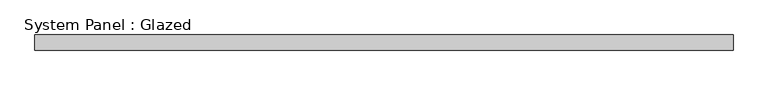
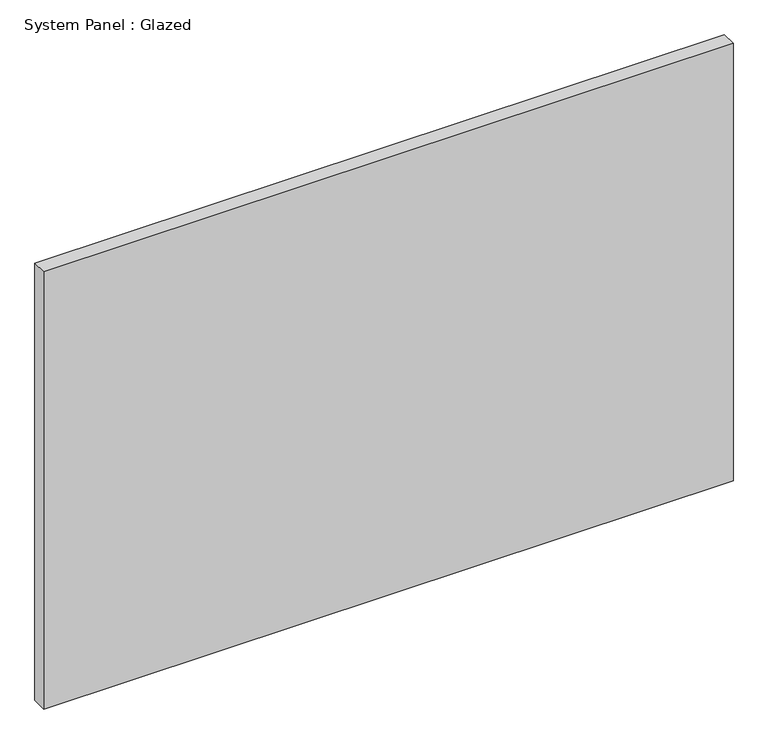
"""IFC4 building model written with IfcOpenShell, lengths in millimetres: plate geometry, System Panel : Glazed."""

from ifc_helpers import new_model, si_unit, origin, origin_with_axes, place, context, project, spatial, polyline, outline, extrude, source, transform, mapped, element, save


def system_panel_glazed_2f542010(model_context):
    return source(origin(), model_context, "Body", "SweptSolid", [
        extrude(outline(polyline([(587.3750001, 19.05), (-587.3750001, 19.05), (-587.3750001, 44.45), (587.3750001, 44.45), (587.3750001, 19.05)])), origin_with_axes(), (0.0, 0.0, 1.0), 787.4),
    ])


if __name__ == "__main__":
    model = new_model("IFC4")
    model_context = context("Model", 3, world=origin())
    ifc_project = project(units=[si_unit("LENGTHUNIT", "METRE", prefix="MILLI")], contexts=[model_context])
    site = spatial("IfcSite", under=ifc_project)
    building = spatial("IfcBuilding", under=site)
    placement = place(None, origin())
    system_panel_glazed_shape = system_panel_glazed_2f542010(model_context)
    element("IfcPlate", 1, ObjectType="System Panel : Glazed", at=placement, inside=building, context=model_context, shape_type="MappedRepresentation", body=[
        mapped(system_panel_glazed_shape, transform((0.0, 0.0, 0.0), x_axis=(1.0, 0.0, 0.0), y_axis=(0.0, 1.0, 0.0), z_axis=(0.0, 0.0, 1.0))),
    ])
    save(model, "model.ifc")

# Revit data of these elements
# Type "System Panel : Glazed"
#   Construction Type Id = "GSP4R"
#   Analytic Construction = "1/8 in Pilkington single glazing"
#   Visual Light Transmittance = 0.9
#   Solar Heat Gain Coefficient = 0.86
#   Heat Transfer Coefficient (U) = 1.18115 BTU/(h·ft²·°F)
#   Define Thermal Properties by = 1
# Element 1 (IfcPlate, "System Panel : Glazed")
#   Materials on its faces: "Glass"
# Materials
#   "Glass": class "Glass", colour RGB 0 128 192, transparency 0.75, Description = "Soda Lime Glass", Cost = 0
